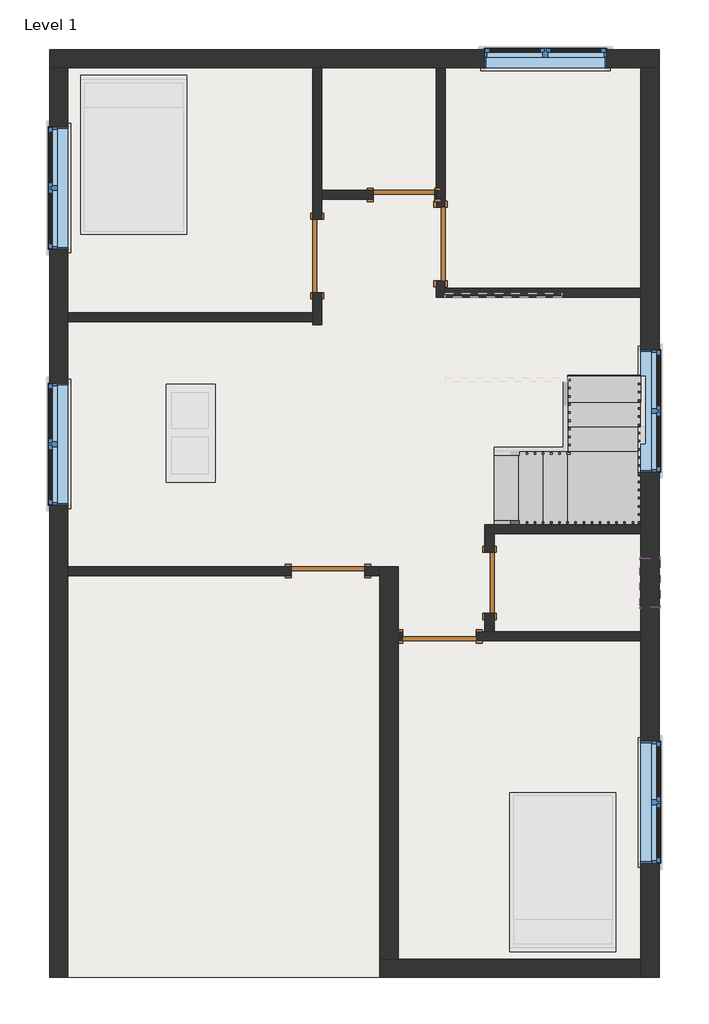
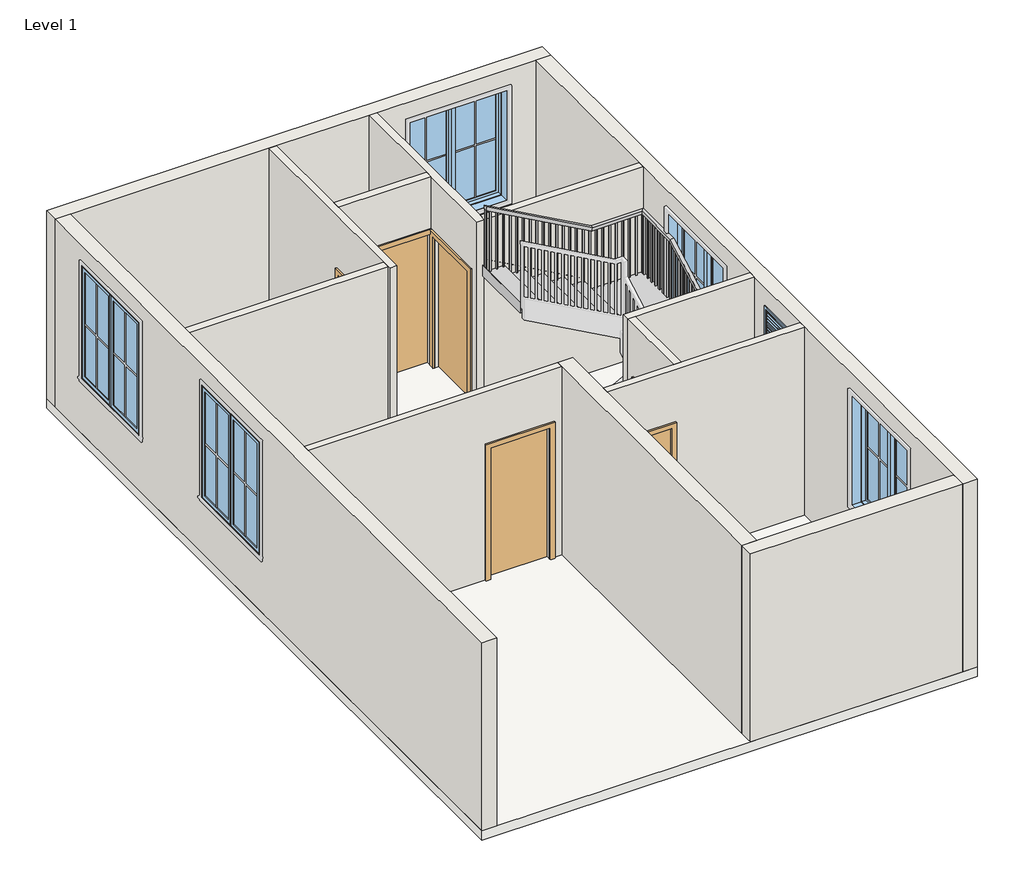
# One storey, part 1 of 2: 14 walls, 6 doors, 6 windows, 1 railing, 1 slab, 1 stair flight.
"""IFC4 building model written with IfcOpenShell, lengths in millimetres."""

from ifc_helpers import new_model, si_unit, frame, origin, origin_with_axes, place, context, project, spatial, polyline, outline, extrude, faceted_brep, transform, mapped, element, save
from components import door_214872d5, door_78caadf7, single_flush_door_3_e5f9f3c4, single_flush_door_3_305aa2a5, stair_flight_7d6782b6, window_casement_double_win_5_f93960c7, window_f2d8fef0

model = new_model("IFC4")

# Units and contexts
model_context = context("Model", 3, world=origin())
ifc_project = project(units=[si_unit("LENGTHUNIT", "METRE", prefix="MILLI")], contexts=[model_context])

# Site, building, storey
site = spatial("IfcSite", under=ifc_project)
building = spatial("IfcBuilding", under=site)
storey = spatial("IfcBuildingStorey", under=building, Name="Level 1", Elevation=0.0)

# Doors
placement = place(None, origin())
door_shape = door_214872d5(model_context)
element("IfcDoor", 1, ObjectType="Single-Flush : DOOR 2'6\"", at=placement, inside=storey, context=model_context, shape_type="MappedRepresentation", body=[
    mapped(door_shape, transform((-185.4325206, 3926.3629493, 0.0), x_axis=(1.0, 0.0, 0.0), y_axis=(0.0, 1.0, 0.0), z_axis=(0.0, 0.0, 1.0))),
])
door_2_shape = door_78caadf7(model_context)
element("IfcDoor", 2, ObjectType="Single-Flush : DOOR 2'6\"", at=placement, inside=storey, context=model_context, shape_type="MappedRepresentation", body=[
    mapped(door_2_shape, transform((881.3674794, -905.9870507, 0.0), x_axis=(0.0, 1.0, 0.0), y_axis=(-1.0, 0.0, 0.0), z_axis=(0.0, 0.0, 1.0))),
])
single_flush_door_3_shape = single_flush_door_3_e5f9f3c4(model_context)
element("IfcDoor", 3, ObjectType="Single-Flush : DOOR 3'", at=placement, inside=storey, context=model_context, shape_type="MappedRepresentation", body=[
    mapped(single_flush_door_3_shape, transform((271.7674794, 3316.7629493, 0.0), x_axis=(0.0, -1.0, 0.0), y_axis=(1.0, 0.0, 0.0), z_axis=(0.0, 0.0, 1.0))),
])
element("IfcDoor", 4, ObjectType="Single-Flush : DOOR 3'", at=placement, inside=storey, context=model_context, shape_type="MappedRepresentation", body=[
    mapped(single_flush_door_3_shape, transform((255.8924794, -1572.7370507, 0.0), x_axis=(-1.0, 0.0, 0.0), y_axis=(0.0, -1.0, 0.0), z_axis=(0.0, 0.0, 1.0))),
])
single_flush_door_3_2_shape = single_flush_door_3_305aa2a5(model_context)
element("IfcDoor", 5, ObjectType="Single-Flush : DOOR 3'", at=placement, inside=storey, context=model_context, shape_type="MappedRepresentation", body=[
    mapped(single_flush_door_3_2_shape, transform((-1264.9325206, 3164.3629493, 0.0), x_axis=(0.0, -1.0, 0.0), y_axis=(1.0, 0.0, 0.0), z_axis=(0.0, 0.0, 1.0))),
])
element("IfcDoor", 6, ObjectType="Single-Flush : DOOR 3'6\"", at=placement, inside=storey, context=model_context, shape_type="MappedRepresentation", body=[
    mapped(single_flush_door_3_shape, transform((-1131.5825206, -759.9370507, 0.0), x_axis=(1.0, 0.0, 0.0), y_axis=(0.0, 1.0, 0.0), z_axis=(0.0, 0.0, 1.0))),
])

# Railing
element("IfcRailing", 7, ObjectType="Handrail - Rectangular", at=placement, inside=storey, context=model_context, shape_type="SolidModel", body=[
    faceted_brep([(938.5174794, -131.2870507, 1083.7333333), (938.5174794, -131.2870507, 1025.620221), (938.5174794, -182.0870507, 1025.620221), (938.5174794, -182.0870507, 1083.7333333), (2005.3174794, -131.2870507, 1676.4), (2018.4810817, -131.2870507, 1625.6), (2018.4810817, -182.0870507, 1625.6), (2005.3174794, -182.0870507, 1676.4), (2716.5174794, -131.2870507, 1676.4), (2716.5174794, -131.2870507, 1625.6), (2767.3174794, -182.0870507, 1625.6), (2767.3174794, -182.0870507, 1676.4), (2716.5174794, 579.9129493, 1676.4), (2716.5174794, 593.0765516, 1625.6), (2767.3174794, 593.0765516, 1625.6), (2767.3174794, 579.9129493, 1676.4), (2716.5174794, 1843.5629493, 2378.4277778), (2716.5174794, 1856.7265516, 2327.6277778), (2767.3174794, 1856.7265516, 2327.6277778), (2767.3174794, 1843.5629493, 2378.4277778), (2716.5174794, 2599.2129493, 2378.4277778), (2716.5174794, 2599.2129493, 2327.6277778), (2767.3174794, 2650.0129493, 2327.6277778), (2767.3174794, 2650.0129493, 2378.4277778), (1960.8674794, 2599.2129493, 2378.4277778), (1947.7038772, 2599.2129493, 2327.6277778), (1947.7038772, 2650.0129493, 2327.6277778), (1960.8674794, 2650.0129493, 2378.4277778), (328.9174794, 2599.2129493, 3285.0666667), (328.9174794, 2650.0129493, 3285.0666667), (328.9174794, 2650.0129493, 3226.9535543), (328.9174794, 2599.2129493, 3226.9535543)], [[[0, 1, 2, 3]], [[1, 0, 4, 5]], [[2, 1, 5, 6]], [[3, 2, 6, 7]], [[0, 3, 7, 4]], [[5, 4, 8, 9]], [[6, 5, 9, 10]], [[7, 6, 10, 11]], [[4, 7, 11, 8]], [[9, 8, 12, 13]], [[10, 9, 13, 14]], [[11, 10, 14, 15]], [[8, 11, 15, 12]], [[13, 12, 16, 17]], [[14, 13, 17, 18]], [[15, 14, 18, 19]], [[12, 15, 19, 16]], [[17, 16, 20, 21]], [[18, 17, 21, 22]], [[19, 18, 22, 23]], [[16, 19, 23, 20]], [[21, 20, 24, 25]], [[22, 21, 25, 26]], [[23, 22, 26, 27]], [[20, 23, 27, 24]], [[28, 29, 30, 31]], [[25, 24, 28, 31]], [[26, 25, 31, 30]], [[27, 26, 30, 29]], [[24, 27, 29, 28]]]),
    extrude(outline(polyline([(3179.3285543, 414.6424794), (3189.9118876, 395.5924794), (2201.3333333, 395.5924794), (2201.3333333, 414.6424794), (3179.3285543, 414.6424794)])), frame((0.0, 2615.0879493, 0.0), z_axis=(0.0, 1.0, 0.0), x_axis=(0.0, 0.0, 1.0)), (0.0, 0.0, 1.0), 19.05),
    extrude(outline(polyline([(3122.8841099, 516.2424794), (3133.4674432, 497.1924794), (2201.3333333, 497.1924794), (2201.3333333, 516.2424794), (3122.8841099, 516.2424794)])), frame((0.0, 2615.0879493, 0.0), z_axis=(0.0, 1.0, 0.0), x_axis=(0.0, 0.0, 1.0)), (0.0, 0.0, 1.0), 19.05),
    extrude(outline(polyline([(3066.4396654, 617.8424794), (3077.0229988, 598.7924794), (2201.3333333, 598.7924794), (2201.3333333, 617.8424794), (3066.4396654, 617.8424794)])), frame((0.0, 2615.0879493, 0.0), z_axis=(0.0, 1.0, 0.0), x_axis=(0.0, 0.0, 1.0)), (0.0, 0.0, 1.0), 19.05),
    extrude(outline(polyline([(3009.995221, 719.4424794), (3020.5785543, 700.3924794), (2032.0, 700.3924794), (2032.0, 719.4424794), (3009.995221, 719.4424794)])), frame((0.0, 2615.0879493, 0.0), z_axis=(0.0, 1.0, 0.0), x_axis=(0.0, 0.0, 1.0)), (0.0, 0.0, 1.0), 19.05),
    extrude(outline(polyline([(2953.5507765, 821.0424794), (2964.1341099, 801.9924794), (2032.0, 801.9924794), (2032.0, 821.0424794), (2953.5507765, 821.0424794)])), frame((0.0, 2615.0879493, 0.0), z_axis=(0.0, 1.0, 0.0), x_axis=(0.0, 0.0, 1.0)), (0.0, 0.0, 1.0), 19.05),
    extrude(outline(polyline([(2897.1063321, 922.6424794), (2907.6896654, 903.5924794), (2032.0, 903.5924794), (2032.0, 922.6424794), (2897.1063321, 922.6424794)])), frame((0.0, 2615.0879493, 0.0), z_axis=(0.0, 1.0, 0.0), x_axis=(0.0, 0.0, 1.0)), (0.0, 0.0, 1.0), 19.05),
    extrude(outline(polyline([(2840.6618876, 1024.2424794), (2851.245221, 1005.1924794), (1862.6666667, 1005.1924794), (1862.6666667, 1024.2424794), (2840.6618876, 1024.2424794)])), frame((0.0, 2615.0879493, 0.0), z_axis=(0.0, 1.0, 0.0), x_axis=(0.0, 0.0, 1.0)), (0.0, 0.0, 1.0), 19.05),
    extrude(outline(polyline([(2784.2174432, 1125.8424794), (2794.8007765, 1106.7924794), (1862.6666667, 1106.7924794), (1862.6666667, 1125.8424794), (2784.2174432, 1125.8424794)])), frame((0.0, 2615.0879493, 0.0), z_axis=(0.0, 1.0, 0.0), x_axis=(0.0, 0.0, 1.0)), (0.0, 0.0, 1.0), 19.05),
    extrude(outline(polyline([(2727.7729988, 1227.4424794), (2738.3563321, 1208.3924794), (1862.6666667, 1208.3924794), (1862.6666667, 1227.4424794), (2727.7729988, 1227.4424794)])), frame((0.0, 2615.0879493, 0.0), z_axis=(0.0, 1.0, 0.0), x_axis=(0.0, 0.0, 1.0)), (0.0, 0.0, 1.0), 19.05),
    extrude(outline(polyline([(2671.3285543, 1329.0424794), (2681.9118876, 1309.9924794), (1693.3333333, 1309.9924794), (1693.3333333, 1329.0424794), (2671.3285543, 1329.0424794)])), frame((0.0, 2615.0879493, 0.0), z_axis=(0.0, 1.0, 0.0), x_axis=(0.0, 0.0, 1.0)), (0.0, 0.0, 1.0), 19.05),
    extrude(outline(polyline([(2614.8841099, 1430.6424794), (2625.4674432, 1411.5924794), (1693.3333333, 1411.5924794), (1693.3333333, 1430.6424794), (2614.8841099, 1430.6424794)])), frame((0.0, 2615.0879493, 0.0), z_axis=(0.0, 1.0, 0.0), x_axis=(0.0, 0.0, 1.0)), (0.0, 0.0, 1.0), 19.05),
    extrude(outline(polyline([(2558.4396654, 1532.2424794), (2569.0229988, 1513.1924794), (1693.3333333, 1513.1924794), (1693.3333333, 1532.2424794), (2558.4396654, 1532.2424794)])), frame((0.0, 2615.0879493, 0.0), z_axis=(0.0, 1.0, 0.0), x_axis=(0.0, 0.0, 1.0)), (0.0, 0.0, 1.0), 19.05),
    extrude(outline(polyline([(2501.995221, 1633.8424794), (2512.5785543, 1614.7924794), (1524.0, 1614.7924794), (1524.0, 1633.8424794), (2501.995221, 1633.8424794)])), frame((0.0, 2615.0879493, 0.0), z_axis=(0.0, 1.0, 0.0), x_axis=(0.0, 0.0, 1.0)), (0.0, 0.0, 1.0), 19.05),
    extrude(outline(polyline([(2445.5507765, 1735.4424794), (2456.1341099, 1716.3924794), (1524.0, 1716.3924794), (1524.0, 1735.4424794), (2445.5507765, 1735.4424794)])), frame((0.0, 2615.0879493, 0.0), z_axis=(0.0, 1.0, 0.0), x_axis=(0.0, 0.0, 1.0)), (0.0, 0.0, 1.0), 19.05),
    extrude(outline(polyline([(2389.1063321, 1837.0424794), (2399.6896654, 1817.9924794), (1524.0, 1817.9924794), (1524.0, 1837.0424794), (2389.1063321, 1837.0424794)])), frame((0.0, 2615.0879493, 0.0), z_axis=(0.0, 1.0, 0.0), x_axis=(0.0, 0.0, 1.0)), (0.0, 0.0, 1.0), 19.05),
    extrude(outline(polyline([(2332.6618876, 1938.6424794), (2343.245221, 1919.5924794), (1354.6666667, 1919.5924794), (1354.6666667, 1938.6424794), (2332.6618876, 1938.6424794)])), frame((0.0, 2615.0879493, 0.0), z_axis=(0.0, 1.0, 0.0), x_axis=(0.0, 0.0, 1.0)), (0.0, 0.0, 1.0), 19.05),
    extrude(outline(polyline([(2040.2424794, 2634.1379493), (2040.2424794, 2615.0879493), (2021.1924794, 2615.0879493), (2021.1924794, 2634.1379493), (2040.2424794, 2634.1379493)])), frame((0.0, 0.0, 1354.6666667), z_axis=(0.0, 0.0, 1.0), x_axis=(1.0, 0.0, 0.0)), (0.0, 0.0, 1.0), 972.9611111),
    extrude(outline(polyline([(2141.8424794, 2634.1379493), (2141.8424794, 2615.0879493), (2122.7924794, 2615.0879493), (2122.7924794, 2634.1379493), (2141.8424794, 2634.1379493)])), frame((0.0, 0.0, 1354.6666667), z_axis=(0.0, 0.0, 1.0), x_axis=(1.0, 0.0, 0.0)), (0.0, 0.0, 1.0), 972.9611111),
    extrude(outline(polyline([(2243.4424794, 2634.1379493), (2243.4424794, 2615.0879493), (2224.3924794, 2615.0879493), (2224.3924794, 2634.1379493), (2243.4424794, 2634.1379493)])), frame((0.0, 0.0, 1354.6666667), z_axis=(0.0, 0.0, 1.0), x_axis=(1.0, 0.0, 0.0)), (0.0, 0.0, 1.0), 972.9611111),
    extrude(outline(polyline([(2345.0424794, 2634.1379493), (2345.0424794, 2615.0879493), (2325.9924794, 2615.0879493), (2325.9924794, 2634.1379493), (2345.0424794, 2634.1379493)])), frame((0.0, 0.0, 1354.6666667), z_axis=(0.0, 0.0, 1.0), x_axis=(1.0, 0.0, 0.0)), (0.0, 0.0, 1.0), 972.9611111),
    extrude(outline(polyline([(2446.6424794, 2634.1379493), (2446.6424794, 2615.0879493), (2427.5924794, 2615.0879493), (2427.5924794, 2634.1379493), (2446.6424794, 2634.1379493)])), frame((0.0, 0.0, 1354.6666667), z_axis=(0.0, 0.0, 1.0), x_axis=(1.0, 0.0, 0.0)), (0.0, 0.0, 1.0), 972.9611111),
    extrude(outline(polyline([(2548.2424794, 2634.1379493), (2548.2424794, 2615.0879493), (2529.1924794, 2615.0879493), (2529.1924794, 2634.1379493), (2548.2424794, 2634.1379493)])), frame((0.0, 0.0, 1354.6666667), z_axis=(0.0, 0.0, 1.0), x_axis=(1.0, 0.0, 0.0)), (0.0, 0.0, 1.0), 972.9611111),
    extrude(outline(polyline([(2649.8424794, 2634.1379493), (2649.8424794, 2615.0879493), (2630.7924794, 2615.0879493), (2630.7924794, 2634.1379493), (2649.8424794, 2634.1379493)])), frame((0.0, 0.0, 1354.6666667), z_axis=(0.0, 0.0, 1.0), x_axis=(1.0, 0.0, 0.0)), (0.0, 0.0, 1.0), 972.9611111),
    extrude(outline(polyline([(2751.4424794, 2576.9879493), (2732.3924794, 2576.9879493), (2732.3924794, 2596.0379493), (2751.4424794, 2596.0379493), (2751.4424794, 2576.9879493)])), frame((0.0, 0.0, 1354.6666667), z_axis=(0.0, 0.0, 1.0), x_axis=(1.0, 0.0, 0.0)), (0.0, 0.0, 1.0), 972.9611111),
    extrude(outline(polyline([(2751.4424794, 2475.3879493), (2732.3924794, 2475.3879493), (2732.3924794, 2494.4379493), (2751.4424794, 2494.4379493), (2751.4424794, 2475.3879493)])), frame((0.0, 0.0, 1354.6666667), z_axis=(0.0, 0.0, 1.0), x_axis=(1.0, 0.0, 0.0)), (0.0, 0.0, 1.0), 972.9611111),
    extrude(outline(polyline([(2751.4424794, 2373.7879493), (2732.3924794, 2373.7879493), (2732.3924794, 2392.8379493), (2751.4424794, 2392.8379493), (2751.4424794, 2373.7879493)])), frame((0.0, 0.0, 1354.6666667), z_axis=(0.0, 0.0, 1.0), x_axis=(1.0, 0.0, 0.0)), (0.0, 0.0, 1.0), 972.9611111),
    extrude(outline(polyline([(2751.4424794, 2272.1879493), (2732.3924794, 2272.1879493), (2732.3924794, 2291.2379493), (2751.4424794, 2291.2379493), (2751.4424794, 2272.1879493)])), frame((0.0, 0.0, 1354.6666667), z_axis=(0.0, 0.0, 1.0), x_axis=(1.0, 0.0, 0.0)), (0.0, 0.0, 1.0), 972.9611111),
    extrude(outline(polyline([(2751.4424794, 2170.5879493), (2732.3924794, 2170.5879493), (2732.3924794, 2189.6379493), (2751.4424794, 2189.6379493), (2751.4424794, 2170.5879493)])), frame((0.0, 0.0, 1354.6666667), z_axis=(0.0, 0.0, 1.0), x_axis=(1.0, 0.0, 0.0)), (0.0, 0.0, 1.0), 972.9611111),
    extrude(outline(polyline([(2751.4424794, 2068.9879493), (2732.3924794, 2068.9879493), (2732.3924794, 2088.0379493), (2751.4424794, 2088.0379493), (2751.4424794, 2068.9879493)])), frame((0.0, 0.0, 1354.6666667), z_axis=(0.0, 0.0, 1.0), x_axis=(1.0, 0.0, 0.0)), (0.0, 0.0, 1.0), 972.9611111),
    extrude(outline(polyline([(2751.4424794, 1967.3879493), (2732.3924794, 1967.3879493), (2732.3924794, 1986.4379493), (2751.4424794, 1986.4379493), (2751.4424794, 1967.3879493)])), frame((0.0, 0.0, 1354.6666667), z_axis=(0.0, 0.0, 1.0), x_axis=(1.0, 0.0, 0.0)), (0.0, 0.0, 1.0), 972.9611111),
    extrude(outline(polyline([(2751.4424794, 1865.7879493), (2732.3924794, 1865.7879493), (2732.3924794, 1884.8379493), (2751.4424794, 1884.8379493), (2751.4424794, 1865.7879493)])), frame((0.0, 0.0, 1354.6666667), z_axis=(0.0, 0.0, 1.0), x_axis=(1.0, 0.0, 0.0)), (0.0, 0.0, 1.0), 972.9611111),
    extrude(outline(polyline([(1764.1879493, 2276.2174432), (1783.2379493, 2286.8007765), (1783.2379493, 1354.6666667), (1764.1879493, 1354.6666667), (1764.1879493, 2276.2174432)])), frame((2732.3924794, 0.0, 0.0), z_axis=(1.0, 0.0, 0.0), x_axis=(0.0, 1.0, 0.0)), (0.0, 0.0, 1.0), 19.05),
    extrude(outline(polyline([(1662.5879493, 2219.7729988), (1681.6379493, 2230.3563321), (1681.6379493, 1354.6666667), (1662.5879493, 1354.6666667), (1662.5879493, 2219.7729988)])), frame((2732.3924794, 0.0, 0.0), z_axis=(1.0, 0.0, 0.0), x_axis=(0.0, 1.0, 0.0)), (0.0, 0.0, 1.0), 19.05),
    extrude(outline(polyline([(1560.9879493, 2163.3285543), (1580.0379493, 2173.9118876), (1580.0379493, 1185.3333333), (1560.9879493, 1185.3333333), (1560.9879493, 2163.3285543)])), frame((2732.3924794, 0.0, 0.0), z_axis=(1.0, 0.0, 0.0), x_axis=(0.0, 1.0, 0.0)), (0.0, 0.0, 1.0), 19.05),
    extrude(outline(polyline([(1459.3879493, 2106.8841099), (1478.4379493, 2117.4674432), (1478.4379493, 1185.3333333), (1459.3879493, 1185.3333333), (1459.3879493, 2106.8841099)])), frame((2732.3924794, 0.0, 0.0), z_axis=(1.0, 0.0, 0.0), x_axis=(0.0, 1.0, 0.0)), (0.0, 0.0, 1.0), 19.05),
    extrude(outline(polyline([(1357.7879493, 2050.4396654), (1376.8379493, 2061.0229988), (1376.8379493, 1185.3333333), (1357.7879493, 1185.3333333), (1357.7879493, 2050.4396654)])), frame((2732.3924794, 0.0, 0.0), z_axis=(1.0, 0.0, 0.0), x_axis=(0.0, 1.0, 0.0)), (0.0, 0.0, 1.0), 19.05),
    extrude(outline(polyline([(1256.1879493, 1993.995221), (1275.2379493, 2004.5785543), (1275.2379493, 1016.0), (1256.1879493, 1016.0), (1256.1879493, 1993.995221)])), frame((2732.3924794, 0.0, 0.0), z_axis=(1.0, 0.0, 0.0), x_axis=(0.0, 1.0, 0.0)), (0.0, 0.0, 1.0), 19.05),
    extrude(outline(polyline([(1154.5879493, 1937.5507765), (1173.6379493, 1948.1341099), (1173.6379493, 1016.0), (1154.5879493, 1016.0), (1154.5879493, 1937.5507765)])), frame((2732.3924794, 0.0, 0.0), z_axis=(1.0, 0.0, 0.0), x_axis=(0.0, 1.0, 0.0)), (0.0, 0.0, 1.0), 19.05),
    extrude(outline(polyline([(1052.9879493, 1881.1063321), (1072.0379493, 1891.6896654), (1072.0379493, 1016.0), (1052.9879493, 1016.0), (1052.9879493, 1881.1063321)])), frame((2732.3924794, 0.0, 0.0), z_axis=(1.0, 0.0, 0.0), x_axis=(0.0, 1.0, 0.0)), (0.0, 0.0, 1.0), 19.05),
    extrude(outline(polyline([(951.3879493, 1824.6618876), (970.4379493, 1835.245221), (970.4379493, 846.6666667), (951.3879493, 846.6666667), (951.3879493, 1824.6618876)])), frame((2732.3924794, 0.0, 0.0), z_axis=(1.0, 0.0, 0.0), x_axis=(0.0, 1.0, 0.0)), (0.0, 0.0, 1.0), 19.05),
    extrude(outline(polyline([(849.7879493, 1768.2174432), (868.8379493, 1778.8007765), (868.8379493, 846.6666667), (849.7879493, 846.6666667), (849.7879493, 1768.2174432)])), frame((2732.3924794, 0.0, 0.0), z_axis=(1.0, 0.0, 0.0), x_axis=(0.0, 1.0, 0.0)), (0.0, 0.0, 1.0), 19.05),
    extrude(outline(polyline([(748.1879493, 1711.7729988), (767.2379493, 1722.3563321), (767.2379493, 846.6666667), (748.1879493, 846.6666667), (748.1879493, 1711.7729988)])), frame((2732.3924794, 0.0, 0.0), z_axis=(1.0, 0.0, 0.0), x_axis=(0.0, 1.0, 0.0)), (0.0, 0.0, 1.0), 19.05),
    extrude(outline(polyline([(646.5879493, 1655.3285543), (665.6379493, 1665.9118876), (665.6379493, 677.3333333), (646.5879493, 677.3333333), (646.5879493, 1655.3285543)])), frame((2732.3924794, 0.0, 0.0), z_axis=(1.0, 0.0, 0.0), x_axis=(0.0, 1.0, 0.0)), (0.0, 0.0, 1.0), 19.05),
    extrude(outline(polyline([(2751.4424794, 544.9879493), (2732.3924794, 544.9879493), (2732.3924794, 564.0379493), (2751.4424794, 564.0379493), (2751.4424794, 544.9879493)])), frame((0.0, 0.0, 677.3333333), z_axis=(0.0, 0.0, 1.0), x_axis=(1.0, 0.0, 0.0)), (0.0, 0.0, 1.0), 948.2666667),
    extrude(outline(polyline([(2751.4424794, 443.3879493), (2732.3924794, 443.3879493), (2732.3924794, 462.4379493), (2751.4424794, 462.4379493), (2751.4424794, 443.3879493)])), frame((0.0, 0.0, 677.3333333), z_axis=(0.0, 0.0, 1.0), x_axis=(1.0, 0.0, 0.0)), (0.0, 0.0, 1.0), 948.2666667),
    extrude(outline(polyline([(2751.4424794, 341.7879493), (2732.3924794, 341.7879493), (2732.3924794, 360.8379493), (2751.4424794, 360.8379493), (2751.4424794, 341.7879493)])), frame((0.0, 0.0, 677.3333333), z_axis=(0.0, 0.0, 1.0), x_axis=(1.0, 0.0, 0.0)), (0.0, 0.0, 1.0), 948.2666667),
    extrude(outline(polyline([(2751.4424794, 240.1879493), (2732.3924794, 240.1879493), (2732.3924794, 259.2379493), (2751.4424794, 259.2379493), (2751.4424794, 240.1879493)])), frame((0.0, 0.0, 677.3333333), z_axis=(0.0, 0.0, 1.0), x_axis=(1.0, 0.0, 0.0)), (0.0, 0.0, 1.0), 948.2666667),
    extrude(outline(polyline([(2751.4424794, 138.5879493), (2732.3924794, 138.5879493), (2732.3924794, 157.6379493), (2751.4424794, 157.6379493), (2751.4424794, 138.5879493)])), frame((0.0, 0.0, 677.3333333), z_axis=(0.0, 0.0, 1.0), x_axis=(1.0, 0.0, 0.0)), (0.0, 0.0, 1.0), 948.2666667),
    extrude(outline(polyline([(2751.4424794, 36.9879493), (2732.3924794, 36.9879493), (2732.3924794, 56.0379493), (2751.4424794, 56.0379493), (2751.4424794, 36.9879493)])), frame((0.0, 0.0, 677.3333333), z_axis=(0.0, 0.0, 1.0), x_axis=(1.0, 0.0, 0.0)), (0.0, 0.0, 1.0), 948.2666667),
    extrude(outline(polyline([(2751.4424794, -64.6120507), (2732.3924794, -64.6120507), (2732.3924794, -45.5620507), (2751.4424794, -45.5620507), (2751.4424794, -64.6120507)])), frame((0.0, 0.0, 677.3333333), z_axis=(0.0, 0.0, 1.0), x_axis=(1.0, 0.0, 0.0)), (0.0, 0.0, 1.0), 948.2666667),
    extrude(outline(polyline([(2656.1924794, -166.2120507), (2656.1924794, -147.1620507), (2675.2424794, -147.1620507), (2675.2424794, -166.2120507), (2656.1924794, -166.2120507)])), frame((0.0, 0.0, 677.3333333), z_axis=(0.0, 0.0, 1.0), x_axis=(1.0, 0.0, 0.0)), (0.0, 0.0, 1.0), 948.2666667),
    extrude(outline(polyline([(2554.5924794, -166.2120507), (2554.5924794, -147.1620507), (2573.6424794, -147.1620507), (2573.6424794, -166.2120507), (2554.5924794, -166.2120507)])), frame((0.0, 0.0, 677.3333333), z_axis=(0.0, 0.0, 1.0), x_axis=(1.0, 0.0, 0.0)), (0.0, 0.0, 1.0), 948.2666667),
    extrude(outline(polyline([(2452.9924794, -166.2120507), (2452.9924794, -147.1620507), (2472.0424794, -147.1620507), (2472.0424794, -166.2120507), (2452.9924794, -166.2120507)])), frame((0.0, 0.0, 677.3333333), z_axis=(0.0, 0.0, 1.0), x_axis=(1.0, 0.0, 0.0)), (0.0, 0.0, 1.0), 948.2666667),
    extrude(outline(polyline([(2351.3924794, -166.2120507), (2351.3924794, -147.1620507), (2370.4424794, -147.1620507), (2370.4424794, -166.2120507), (2351.3924794, -166.2120507)])), frame((0.0, 0.0, 677.3333333), z_axis=(0.0, 0.0, 1.0), x_axis=(1.0, 0.0, 0.0)), (0.0, 0.0, 1.0), 948.2666667),
    extrude(outline(polyline([(2249.7924794, -166.2120507), (2249.7924794, -147.1620507), (2268.8424794, -147.1620507), (2268.8424794, -166.2120507), (2249.7924794, -166.2120507)])), frame((0.0, 0.0, 677.3333333), z_axis=(0.0, 0.0, 1.0), x_axis=(1.0, 0.0, 0.0)), (0.0, 0.0, 1.0), 948.2666667),
    extrude(outline(polyline([(2148.1924794, -166.2120507), (2148.1924794, -147.1620507), (2167.2424794, -147.1620507), (2167.2424794, -166.2120507), (2148.1924794, -166.2120507)])), frame((0.0, 0.0, 677.3333333), z_axis=(0.0, 0.0, 1.0), x_axis=(1.0, 0.0, 0.0)), (0.0, 0.0, 1.0), 948.2666667),
    extrude(outline(polyline([(2046.5924794, -166.2120507), (2046.5924794, -147.1620507), (2065.6424794, -147.1620507), (2065.6424794, -166.2120507), (2046.5924794, -166.2120507)])), frame((0.0, 0.0, 677.3333333), z_axis=(0.0, 0.0, 1.0), x_axis=(1.0, 0.0, 0.0)), (0.0, 0.0, 1.0), 948.2666667),
    extrude(outline(polyline([(1595.3563321, 1964.0424794), (1584.7729988, 1944.9924794), (677.3333333, 1944.9924794), (677.3333333, 1964.0424794), (1595.3563321, 1964.0424794)])), frame((0.0, -166.2120507, 0.0), z_axis=(0.0, 1.0, 0.0), x_axis=(0.0, 0.0, 1.0)), (0.0, 0.0, 1.0), 19.05),
    extrude(outline(polyline([(1538.9118876, 1862.4424794), (1528.3285543, 1843.3924794), (677.3333333, 1843.3924794), (677.3333333, 1862.4424794), (1538.9118876, 1862.4424794)])), frame((0.0, -166.2120507, 0.0), z_axis=(0.0, 1.0, 0.0), x_axis=(0.0, 0.0, 1.0)), (0.0, 0.0, 1.0), 19.05),
    extrude(outline(polyline([(1482.4674432, 1760.8424794), (1471.8841099, 1741.7924794), (508.0, 1741.7924794), (508.0, 1760.8424794), (1482.4674432, 1760.8424794)])), frame((0.0, -166.2120507, 0.0), z_axis=(0.0, 1.0, 0.0), x_axis=(0.0, 0.0, 1.0)), (0.0, 0.0, 1.0), 19.05),
    extrude(outline(polyline([(1426.0229988, 1659.2424794), (1415.4396654, 1640.1924794), (508.0, 1640.1924794), (508.0, 1659.2424794), (1426.0229988, 1659.2424794)])), frame((0.0, -166.2120507, 0.0), z_axis=(0.0, 1.0, 0.0), x_axis=(0.0, 0.0, 1.0)), (0.0, 0.0, 1.0), 19.05),
    extrude(outline(polyline([(1369.5785543, 1557.6424794), (1358.995221, 1538.5924794), (508.0, 1538.5924794), (508.0, 1557.6424794), (1369.5785543, 1557.6424794)])), frame((0.0, -166.2120507, 0.0), z_axis=(0.0, 1.0, 0.0), x_axis=(0.0, 0.0, 1.0)), (0.0, 0.0, 1.0), 19.05),
    extrude(outline(polyline([(1313.1341099, 1456.0424794), (1302.5507765, 1436.9924794), (338.6666667, 1436.9924794), (338.6666667, 1456.0424794), (1313.1341099, 1456.0424794)])), frame((0.0, -166.2120507, 0.0), z_axis=(0.0, 1.0, 0.0), x_axis=(0.0, 0.0, 1.0)), (0.0, 0.0, 1.0), 19.05),
    extrude(outline(polyline([(1256.6896654, 1354.4424794), (1246.1063321, 1335.3924794), (338.6666667, 1335.3924794), (338.6666667, 1354.4424794), (1256.6896654, 1354.4424794)])), frame((0.0, -166.2120507, 0.0), z_axis=(0.0, 1.0, 0.0), x_axis=(0.0, 0.0, 1.0)), (0.0, 0.0, 1.0), 19.05),
    extrude(outline(polyline([(1200.245221, 1252.8424794), (1189.6618876, 1233.7924794), (338.6666667, 1233.7924794), (338.6666667, 1252.8424794), (1200.245221, 1252.8424794)])), frame((0.0, -166.2120507, 0.0), z_axis=(0.0, 1.0, 0.0), x_axis=(0.0, 0.0, 1.0)), (0.0, 0.0, 1.0), 19.05),
    extrude(outline(polyline([(1143.8007765, 1151.2424794), (1133.2174432, 1132.1924794), (169.3333333, 1132.1924794), (169.3333333, 1151.2424794), (1143.8007765, 1151.2424794)])), frame((0.0, -166.2120507, 0.0), z_axis=(0.0, 1.0, 0.0), x_axis=(0.0, 0.0, 1.0)), (0.0, 0.0, 1.0), 19.05),
    extrude(outline(polyline([(1087.3563321, 1049.6424794), (1076.7729988, 1030.5924794), (169.3333333, 1030.5924794), (169.3333333, 1049.6424794), (1087.3563321, 1049.6424794)])), frame((0.0, -166.2120507, 0.0), z_axis=(0.0, 1.0, 0.0), x_axis=(0.0, 0.0, 1.0)), (0.0, 0.0, 1.0), 19.05),
    extrude(outline(polyline([(2751.4424794, 2615.0879493), (2732.3924794, 2615.0879493), (2732.3924794, 2634.1379493), (2751.4424794, 2634.1379493), (2751.4424794, 2615.0879493)])), frame((0.0, 0.0, 1354.6666667), z_axis=(0.0, 0.0, 1.0), x_axis=(1.0, 0.0, 0.0)), (0.0, 0.0, 1.0), 972.9611111),
    extrude(outline(polyline([(2732.3924794, -166.2120507), (2732.3924794, -147.1620507), (2751.4424794, -147.1620507), (2751.4424794, -166.2120507), (2732.3924794, -166.2120507)])), frame((0.0, 0.0, 677.3333333), z_axis=(0.0, 0.0, 1.0), x_axis=(1.0, 0.0, 0.0)), (0.0, 0.0, 1.0), 948.2666667),
    extrude(outline(polyline([(3216.370221, 347.9674794), (3226.9535543, 328.9174794), (2201.3333333, 328.9174794), (2201.3333333, 347.9674794), (3216.370221, 347.9674794)])), frame((0.0, 2615.0879493, 0.0), z_axis=(0.0, 1.0, 0.0), x_axis=(0.0, 0.0, 1.0)), (0.0, 0.0, 1.0), 19.05),
    extrude(outline(polyline([(1036.2035543, 957.5674794), (1025.620221, 938.5174794), (169.3333333, 938.5174794), (169.3333333, 957.5674794), (1036.2035543, 957.5674794)])), frame((0.0, -166.2120507, 0.0), z_axis=(0.0, 1.0, 0.0), x_axis=(0.0, 0.0, 1.0)), (0.0, 0.0, 1.0), 19.05),
])

# Slab
element("IfcSlab", 8, ObjectType="FLOOR 6\"", at=placement, inside=storey, context=model_context, shape_type="SweptSolid", body=[
    extrude(outline(polyline([(2995.9174794, 5736.1129493), (2995.9174794, -5820.8870507), (-4598.6825206, -5820.8870507), (-4598.6825206, 5736.1129493), (2995.9174794, 5736.1129493)])), frame((0.0, 0.0, -152.4), z_axis=(0.0, 0.0, 1.0), x_axis=(1.0, 0.0, 0.0)), (0.0, 0.0, 1.0), 152.4),
])

# Stair flight
stair_flight_shape = stair_flight_7d6782b6(model_context)
element("IfcStairFlight", 9, ObjectType="2\" Tread 1\" Nosing 1/4\" Riser", at=placement, inside=storey, context=model_context, shape_type="MappedRepresentation", body=[
    mapped(stair_flight_shape, transform((0.0, 0.0, 0.0), x_axis=(1.0, 0.0, 0.0), y_axis=(0.0, 1.0, 0.0), z_axis=(0.0, 0.0, 1.0))),
])

# Walls
element("IfcWall", 10, at=placement, inside=storey, context=model_context, shape_type="Brep", body=[
    faceted_brep([(-1322.0825206, 2707.1629493, 2133.6), (-1322.0825206, 2707.1629493, 0.0), (-1322.0825206, 2459.5129493, 0.0), (-1322.0825206, 2345.2129493, 0.0), (-1322.0825206, 2307.1129493, 0.0), (-1322.0825206, 2307.1129493, 3048.0), (-1322.0825206, 2345.2129493, 3048.0), (-1322.0825206, 2459.5129493, 3048.0), (-1322.0825206, 5507.5129493, 3048.0), (-1322.0825206, 5507.5129493, 0.0), (-1322.0825206, 3621.5629493, 0.0), (-1322.0825206, 3621.5629493, 2133.6), (-1207.7825206, 2307.1129493, 0.0), (-1207.7825206, 2707.1629493, 0.0), (-1207.7825206, 2707.1629493, 2133.6), (-1207.7825206, 3621.5629493, 2133.6), (-1207.7825206, 3621.5629493, 0.0), (-1207.7825206, 3869.2129493, 0.0), (-1207.7825206, 3983.5129493, 0.0), (-1207.7825206, 5507.5129493, 0.0), (-1207.7825206, 5507.5129493, 3048.0), (-1207.7825206, 3983.5129493, 3048.0), (-1207.7825206, 3869.2129493, 3048.0), (-1207.7825206, 2307.1129493, 3048.0)], [[[0, 1, 2, 3, 4, 5, 6, 7, 8, 9, 10, 11]], [[12, 13, 14, 15, 16, 17, 18, 19, 20, 21, 22, 23]], [[10, 9, 19, 18, 17, 16]], [[4, 3, 2, 1, 13, 12]], [[5, 4, 12, 23]], [[9, 8, 20, 19]], [[14, 13, 1, 0]], [[15, 14, 0, 11]], [[16, 15, 11, 10]], [[8, 7, 6, 5, 23, 22, 21, 20]]]),
])
element("IfcWall", 11, at=placement, inside=storey, context=model_context, shape_type="SweptSolid", body=[
    extrude(outline(polyline([(-1322.0825206, 2345.2129493), (-4370.0825206, 2345.2129493), (-4370.0825206, 2459.5129493), (-1322.0825206, 2459.5129493), (-1322.0825206, 2345.2129493)])), origin_with_axes(), (0.0, 0.0, 1.0), 3048.0),
])
element("IfcWall", 12, at=placement, inside=storey, context=model_context, shape_type="SweptSolid", body=[
    extrude(outline(polyline([(2133.6, 195.5674794), (0.0, 195.5674794), (0.0, 214.6174794), (3048.0, 214.6174794), (3048.0, -1207.7825206), (0.0, -1207.7825206), (0.0, -566.4325206), (2133.6, -566.4325206), (2133.6, 195.5674794)])), frame((0.0, 3869.2129493, 0.0), z_axis=(0.0, 1.0, 0.0), x_axis=(0.0, 0.0, 1.0)), (0.0, 0.0, 1.0), 114.3),
])
element("IfcWall", 13, at=placement, inside=storey, context=model_context, shape_type="Brep", body=[
    faceted_brep([(214.6174794, 2859.5629493, 2133.6), (214.6174794, 2859.5629493, 0.0), (214.6174794, 2650.0129493, 0.0), (214.6174794, 2650.0129493, 3048.0), (214.6174794, 3869.2129493, 3048.0), (214.6174794, 3983.5129493, 3048.0), (214.6174794, 5507.5129493, 3048.0), (214.6174794, 5507.5129493, 0.0), (214.6174794, 3983.5129493, 0.0), (214.6174794, 3869.2129493, 0.0), (214.6174794, 3773.9629493, 0.0), (214.6174794, 3773.9629493, 2133.6), (328.9174794, 2650.0129493, 0.0), (328.9174794, 2764.3129493, 0.0), (328.9174794, 2859.5629493, 0.0), (328.9174794, 2859.5629493, 2133.6), (328.9174794, 3773.9629493, 2133.6), (328.9174794, 3773.9629493, 0.0), (328.9174794, 5507.5129493, 0.0), (328.9174794, 5507.5129493, 3048.0), (328.9174794, 2764.3129493, 3048.0), (328.9174794, 2650.0129493, 3048.0)], [[[0, 1, 2, 3, 4, 5, 6, 7, 8, 9, 10, 11]], [[12, 13, 14, 15, 16, 17, 18, 19, 20, 21]], [[2, 1, 14, 13, 12]], [[10, 9, 8, 7, 18, 17]], [[7, 6, 19, 18]], [[3, 2, 12, 21]], [[15, 14, 1, 0]], [[16, 15, 0, 11]], [[17, 16, 11, 10]], [[6, 5, 4, 3, 21, 20, 19]]]),
])
element("IfcWall", 14, at=placement, inside=storey, context=model_context, shape_type="SweptSolid", body=[
    extrude(outline(polyline([(2767.3174794, 2650.0129493), (328.9174794, 2650.0129493), (328.9174794, 2764.3129493), (2767.3174794, 2764.3129493), (2767.3174794, 2650.0129493)])), origin_with_axes(), (0.0, 0.0, 1.0), 3048.0),
])
element("IfcWall", 15, at=placement, inside=storey, context=model_context, shape_type="Brep", body=[
    faceted_brep([(2767.3174794, -182.0870507, 0.0), (824.2174794, -182.0870507, 0.0), (824.2174794, -182.0870507, 3048.0), (2767.3174794, -182.0870507, 3048.0), (2767.3174794, -296.3870507, 0.0), (2767.3174794, -296.3870507, 3048.0), (938.5174794, -296.3870507, 3048.0), (824.2174794, -296.3870507, 3048.0), (824.2174794, -296.3870507, 0.0), (938.5174794, -296.3870507, 0.0)], [[[0, 1, 2, 3]], [[4, 5, 6, 7, 8, 9]], [[1, 0, 4, 9, 8]], [[0, 3, 5, 4]], [[2, 1, 8, 7]], [[3, 2, 7, 6, 5]]]),
])
element("IfcWall", 16, at=placement, inside=storey, context=model_context, shape_type="SweptSolid", body=[
    extrude(outline(polyline([(-296.3870507, 0.0), (-524.9870507, 0.0), (-524.9870507, 2133.6), (-1286.9870507, 2133.6), (-1286.9870507, 0.0), (-1515.5870507, 0.0), (-1515.5870507, 3048.0), (-296.3870507, 3048.0), (-296.3870507, 0.0)])), frame((824.2174794, 0.0, 0.0), z_axis=(1.0, 0.0, 0.0), x_axis=(0.0, 1.0, 0.0)), (0.0, 0.0, 1.0), 114.3),
])
element("IfcWall", 17, at=placement, inside=storey, context=model_context, shape_type="Brep", body=[
    faceted_brep([(-201.3075206, -1515.5870507, 2133.6), (-201.3075206, -1515.5870507, 0.0), (-255.2825206, -1515.5870507, 0.0), (-255.2825206, -1515.5870507, 3048.0), (824.2174794, -1515.5870507, 3048.0), (938.5174794, -1515.5870507, 3048.0), (2767.3174794, -1515.5870507, 3048.0), (2767.3174794, -1515.5870507, 0.0), (938.5174794, -1515.5870507, 0.0), (824.2174794, -1515.5870507, 0.0), (713.0924794, -1515.5870507, 0.0), (713.0924794, -1515.5870507, 2133.6), (-255.2825206, -1629.8870507, 0.0), (-201.3075206, -1629.8870507, 0.0), (-201.3075206, -1629.8870507, 2133.6), (713.0924794, -1629.8870507, 2133.6), (713.0924794, -1629.8870507, 0.0), (2767.3174794, -1629.8870507, 0.0), (2767.3174794, -1629.8870507, 3048.0), (-255.2825206, -1629.8870507, 3048.0)], [[[0, 1, 2, 3, 4, 5, 6, 7, 8, 9, 10, 11]], [[12, 13, 14, 15, 16, 17, 18, 19]], [[2, 1, 13, 12]], [[10, 9, 8, 7, 17, 16]], [[7, 6, 18, 17]], [[3, 2, 12, 19]], [[14, 13, 1, 0]], [[15, 14, 0, 11]], [[16, 15, 11, 10]], [[6, 5, 4, 3, 19, 18]]]),
])
element("IfcWall", 18, at=placement, inside=storey, context=model_context, shape_type="SweptSolid", body=[
    extrude(outline(polyline([(2133.6, -674.3825206), (0.0, -674.3825206), (0.0, -483.8825206), (3048.0, -483.8825206), (3048.0, -4370.0825206), (0.0, -4370.0825206), (0.0, -1588.7825206), (2133.6, -1588.7825206), (2133.6, -674.3825206)])), frame((0.0, -817.0870507, 0.0), z_axis=(0.0, 1.0, 0.0), x_axis=(0.0, 0.0, 1.0)), (0.0, 0.0, 1.0), 114.3),
])
element("IfcWall", 19, ObjectType="WALL 9\"", at=placement, inside=storey, context=model_context, shape_type="Brep", body=[
    faceted_brep([(-4598.6825206, 5507.5129493, 0.0), (-4370.0825206, 5507.5129493, 0.0), (-1322.0825206, 5507.5129493, 0.0), (-1207.7825206, 5507.5129493, 0.0), (214.6174794, 5507.5129493, 0.0), (328.9174794, 5507.5129493, 0.0), (2767.3174794, 5507.5129493, 0.0), (2995.9174794, 5507.5129493, 0.0), (2995.9174794, 5507.5129493, 3048.0), (2767.3174794, 5507.5129493, 3048.0), (328.9174794, 5507.5129493, 3048.0), (214.6174794, 5507.5129493, 3048.0), (-1207.7825206, 5507.5129493, 3048.0), (-1322.0825206, 5507.5129493, 3048.0), (-4370.0825206, 5507.5129493, 3048.0), (-4598.6825206, 5507.5129493, 3048.0), (2338.6924794, 5507.5129493, 2743.2), (2338.6924794, 5507.5129493, 914.4), (814.6924794, 5507.5129493, 914.4), (814.6924794, 5507.5129493, 2743.2), (-4598.6825206, 5736.1129493, 0.0), (-4598.6825206, 5736.1129493, 3048.0), (2995.9174794, 5736.1129493, 3048.0), (2995.9174794, 5736.1129493, 0.0), (2338.6924794, 5736.1129493, 2743.2), (814.6924794, 5736.1129493, 2743.2), (814.6924794, 5736.1129493, 914.4), (2338.6924794, 5736.1129493, 914.4)], [[[0, 1, 2, 3, 4, 5, 6, 7, 8, 9, 10, 11, 12, 13, 14, 15], [16, 17, 18, 19]], [[20, 21, 22, 23], [24, 25, 26, 27]], [[7, 6, 5, 4, 3, 2, 1, 0, 20, 23]], [[8, 7, 23, 22]], [[0, 15, 21, 20]], [[17, 16, 24, 27]], [[18, 17, 27, 26]], [[19, 18, 26, 25]], [[16, 19, 25, 24]], [[15, 14, 13, 12, 11, 10, 9, 8, 22, 21]]]),
])
element("IfcWall", 20, ObjectType="WALL 9\"", at=placement, inside=storey, context=model_context, shape_type="Brep", body=[
    faceted_brep([(2767.3174794, 5507.5129493, 0.0), (2767.3174794, 2764.3129493, 0.0), (2767.3174794, 2650.0129493, 0.0), (2767.3174794, -182.0870507, 0.0), (2767.3174794, -296.3870507, 0.0), (2767.3174794, -1515.5870507, 0.0), (2767.3174794, -1629.8870507, 0.0), (2767.3174794, -5592.2870507, 0.0), (2767.3174794, -5820.8870507, 0.0), (2767.3174794, -5820.8870507, 3048.0), (2767.3174794, -5592.2870507, 3048.0), (2767.3174794, -1629.8870507, 3048.0), (2767.3174794, -1515.5870507, 3048.0), (2767.3174794, -296.3870507, 3048.0), (2767.3174794, -182.0870507, 3048.0), (2767.3174794, 2650.0129493, 3048.0), (2767.3174794, 2764.3129493, 3048.0), (2767.3174794, 5507.5129493, 3048.0), (2767.3174794, 471.9629493, 2743.2), (2767.3174794, 471.9629493, 914.4), (2767.3174794, 1995.9629493, 914.4), (2767.3174794, 1995.9629493, 2743.2), (2767.3174794, -4401.6620507, 2743.2), (2767.3174794, -4401.6620507, 914.4), (2767.3174794, -2877.6620507, 914.4), (2767.3174794, -2877.6620507, 2743.2), (2767.3174794, -1210.7870507, 2743.2), (2767.3174794, -1210.7870507, 2133.6), (2767.3174794, -601.1870507, 2133.6), (2767.3174794, -601.1870507, 2743.2), (2995.9174794, 5507.5129493, 0.0), (2995.9174794, 5507.5129493, 3048.0), (2995.9174794, -5820.8870507, 3048.0), (2995.9174794, -5820.8870507, 0.0), (2995.9174794, 471.9629493, 2743.2), (2995.9174794, 1995.9629493, 2743.2), (2995.9174794, 1995.9629493, 914.4), (2995.9174794, 471.9629493, 914.4), (2995.9174794, -4401.6620507, 2743.2), (2995.9174794, -2877.6620507, 2743.2), (2995.9174794, -2877.6620507, 914.4), (2995.9174794, -4401.6620507, 914.4), (2995.9174794, -1210.7870507, 2743.2), (2995.9174794, -601.1870507, 2743.2), (2995.9174794, -601.1870507, 2133.6), (2995.9174794, -1210.7870507, 2133.6)], [[[0, 1, 2, 3, 4, 5, 6, 7, 8, 9, 10, 11, 12, 13, 14, 15, 16, 17], [18, 19, 20, 21], [22, 23, 24, 25], [26, 27, 28, 29]], [[30, 31, 32, 33], [34, 35, 36, 37], [38, 39, 40, 41], [42, 43, 44, 45]], [[8, 7, 6, 5, 4, 3, 2, 1, 0, 30, 33]], [[0, 17, 31, 30]], [[9, 8, 33, 32]], [[19, 18, 34, 37]], [[20, 19, 37, 36]], [[21, 20, 36, 35]], [[18, 21, 35, 34]], [[23, 22, 38, 41]], [[24, 23, 41, 40]], [[25, 24, 40, 39]], [[22, 25, 39, 38]], [[27, 26, 42, 45]], [[28, 27, 45, 44]], [[29, 28, 44, 43]], [[26, 29, 43, 42]], [[17, 16, 15, 14, 13, 12, 11, 10, 9, 32, 31]]]),
])
element("IfcWall", 21, ObjectType="WALL 9\"", at=placement, inside=storey, context=model_context, shape_type="Brep", body=[
    faceted_brep([(2767.3174794, -5592.2870507, 0.0), (-255.2825206, -5592.2870507, 0.0), (-483.8825206, -5592.2870507, 0.0), (-483.8825206, -5592.2870507, 3048.0), (-255.2825206, -5592.2870507, 3048.0), (2767.3174794, -5592.2870507, 3048.0), (2767.3174794, -5820.8870507, 0.0), (2767.3174794, -5820.8870507, 3048.0), (-483.8825206, -5820.8870507, 3048.0), (-483.8825206, -5820.8870507, 0.0)], [[[0, 1, 2, 3, 4, 5]], [[6, 7, 8, 9]], [[2, 1, 0, 6, 9]], [[0, 5, 7, 6]], [[3, 2, 9, 8]], [[5, 4, 3, 8, 7]]]),
])
element("IfcWall", 22, ObjectType="WALL 9\"", at=placement, inside=storey, context=model_context, shape_type="Brep", body=[
    faceted_brep([(-255.2825206, -5592.2870507, 0.0), (-255.2825206, -1629.8870507, 0.0), (-255.2825206, -1515.5870507, 0.0), (-255.2825206, -702.7870507, 0.0), (-255.2825206, -702.7870507, 3048.0), (-255.2825206, -1515.5870507, 3048.0), (-255.2825206, -1629.8870507, 3048.0), (-255.2825206, -5592.2870507, 3048.0), (-483.8825206, -5592.2870507, 0.0), (-483.8825206, -5592.2870507, 3048.0), (-483.8825206, -817.0870507, 3048.0), (-483.8825206, -702.7870507, 3048.0), (-483.8825206, -702.7870507, 0.0), (-483.8825206, -817.0870507, 0.0)], [[[0, 1, 2, 3, 4, 5, 6, 7]], [[8, 9, 10, 11, 12, 13]], [[3, 2, 1, 0, 8, 13, 12]], [[0, 7, 9, 8]], [[4, 3, 12, 11]], [[7, 6, 5, 4, 11, 10, 9]]]),
])
element("IfcWall", 23, ObjectType="WALL 9\"", at=placement, inside=storey, context=model_context, shape_type="Brep", body=[
    faceted_brep([(-4370.0825206, -5820.8870507, 0.0), (-4370.0825206, -817.0870507, 0.0), (-4370.0825206, -702.7870507, 0.0), (-4370.0825206, 2345.2129493, 0.0), (-4370.0825206, 2459.5129493, 0.0), (-4370.0825206, 5507.5129493, 0.0), (-4370.0825206, 5507.5129493, 3048.0), (-4370.0825206, 2459.5129493, 3048.0), (-4370.0825206, 2345.2129493, 3048.0), (-4370.0825206, -702.7870507, 3048.0), (-4370.0825206, -817.0870507, 3048.0), (-4370.0825206, -5820.8870507, 3048.0), (-4370.0825206, 1583.2129493, 2743.2), (-4370.0825206, 1583.2129493, 914.4), (-4370.0825206, 59.2129493, 914.4), (-4370.0825206, 59.2129493, 2743.2), (-4370.0825206, 4774.0879493, 2743.2), (-4370.0825206, 4774.0879493, 914.4), (-4370.0825206, 3250.0879493, 914.4), (-4370.0825206, 3250.0879493, 2743.2), (-4598.6825206, -5820.8870507, 0.0), (-4598.6825206, -5820.8870507, 3048.0), (-4598.6825206, 5507.5129493, 3048.0), (-4598.6825206, 5507.5129493, 0.0), (-4598.6825206, 1583.2129493, 2743.2), (-4598.6825206, 59.2129493, 2743.2), (-4598.6825206, 59.2129493, 914.4), (-4598.6825206, 1583.2129493, 914.4), (-4598.6825206, 4774.0879493, 2743.2), (-4598.6825206, 3250.0879493, 2743.2), (-4598.6825206, 3250.0879493, 914.4), (-4598.6825206, 4774.0879493, 914.4)], [[[0, 1, 2, 3, 4, 5, 6, 7, 8, 9, 10, 11], [12, 13, 14, 15], [16, 17, 18, 19]], [[20, 21, 22, 23], [24, 25, 26, 27], [28, 29, 30, 31]], [[5, 4, 3, 2, 1, 0, 20, 23]], [[0, 11, 21, 20]], [[6, 5, 23, 22]], [[13, 12, 24, 27]], [[14, 13, 27, 26]], [[15, 14, 26, 25]], [[12, 15, 25, 24]], [[17, 16, 28, 31]], [[18, 17, 31, 30]], [[19, 18, 30, 29]], [[16, 19, 29, 28]], [[11, 10, 9, 8, 7, 6, 22, 21]]]),
])

# Windows
window_casement_double_win_5_shape = window_casement_double_win_5_f93960c7(model_context)
element("IfcWindow", 24, ObjectType="Window-Casement-Double : WIN 5'", at=placement, inside=storey, context=model_context, shape_type="MappedRepresentation", body=[
    mapped(window_casement_double_win_5_shape, transform((-4484.3825206, 821.2129493, 0.0), x_axis=(0.0, 1.0, 0.0), y_axis=(-1.0, 0.0, 0.0), z_axis=(0.0, 0.0, 1.0))),
])
element("IfcWindow", 25, ObjectType="Window-Casement-Double : WIN 5'", at=placement, inside=storey, context=model_context, shape_type="MappedRepresentation", body=[
    mapped(window_casement_double_win_5_shape, transform((-4484.3825206, 4012.0879493, 0.0), x_axis=(0.0, 1.0, 0.0), y_axis=(-1.0, 0.0, 0.0), z_axis=(0.0, 0.0, 1.0))),
])
element("IfcWindow", 26, ObjectType="Window-Casement-Double : WIN 5'", at=placement, inside=storey, context=model_context, shape_type="MappedRepresentation", body=[
    mapped(window_casement_double_win_5_shape, transform((1576.6924794, 5621.8129493, 0.0), x_axis=(1.0, 0.0, 0.0), y_axis=(0.0, 1.0, 0.0), z_axis=(0.0, 0.0, 1.0))),
])
element("IfcWindow", 27, ObjectType="Window-Casement-Double : WIN 5'", at=placement, inside=storey, context=model_context, shape_type="MappedRepresentation", body=[
    mapped(window_casement_double_win_5_shape, transform((2881.6174794, 1233.9629493, 0.0), x_axis=(0.0, -1.0, 0.0), y_axis=(1.0, 0.0, 0.0), z_axis=(0.0, 0.0, 1.0))),
])
element("IfcWindow", 28, ObjectType="Window-Casement-Double : WIN 5'", at=placement, inside=storey, context=model_context, shape_type="MappedRepresentation", body=[
    mapped(window_casement_double_win_5_shape, transform((2881.6174794, -3639.6620507, 0.0), x_axis=(0.0, -1.0, 0.0), y_axis=(1.0, 0.0, 0.0), z_axis=(0.0, 0.0, 1.0))),
])
window_shape = window_f2d8fef0(model_context)
element("IfcWindow", 29, ObjectType="Window-Louvers : 24\" x 24\"", at=placement, inside=storey, context=model_context, shape_type="MappedRepresentation", body=[
    mapped(window_shape, transform((2875.2674794, -905.9870507, 1219.2), x_axis=(0.0, 1.0, 0.0), y_axis=(-1.0, 0.0, 0.0), z_axis=(0.0, 0.0, 1.0))),
])

save(model, "model.ifc")

# Revit data of these elements
# Type "Single-Flush : DOOR 2'6\""
#   Type Mark = "10"
#   Construction Type Id = "MDOOR"
#   Assembly Code = "C1020"
#   Analytic Construction = "Metal"
#   Thickness = 0' - 2"
#   Heat Transfer Coefficient (U) = 0.651978 BTU/(h·ft²·°F)
#   Height = 7' - 0"
#   Trim Projection Ext = 0' - 1"
#   Trim Projection Int = 0' - 1"
#   Trim Width = 0' - 3"
#   Width = 2' - 6"
#   Define Thermal Properties by = 1
#   Door Material = Door - Panel
#   Frame Material = Door - Frame
#   Visual Light Transmittance = 0
#   Solar Heat Gain Coefficient = 0
#   Function = (empty or 0)
#   Wall Closure = (empty or 0)
# Type "Single-Flush : DOOR 3'"
#   Type Mark = "9"
#   Construction Type Id = "MDOOR"
#   Assembly Code = "C1020"
#   Analytic Construction = "Metal"
#   Thickness = 0' - 2"
#   Heat Transfer Coefficient (U) = 0.651978 BTU/(h·ft²·°F)
#   Height = 7' - 0"
#   Trim Projection Ext = 0' - 1"
#   Trim Projection Int = 0' - 1"
#   Trim Width = 0' - 3"
#   Width = 3' - 0"
#   Define Thermal Properties by = 1
#   Door Material = Door - Panel
#   Frame Material = Door - Frame
#   Visual Light Transmittance = 0
#   Solar Heat Gain Coefficient = 0
#   Function = (empty or 0)
#   Wall Closure = (empty or 0)
# Type "Single-Flush : DOOR 3'6\""
#   Type Mark = "8"
#   Construction Type Id = "MDOOR"
#   Assembly Code = "C1020"
#   Analytic Construction = "Metal"
#   Thickness = 0' - 2"
#   Heat Transfer Coefficient (U) = 0.651978 BTU/(h·ft²·°F)
#   Height = 7' - 0"
#   Trim Projection Ext = 0' - 1"
#   Trim Projection Int = 0' - 1"
#   Trim Width = 0' - 3"
#   Width = 3' - 0"
#   Define Thermal Properties by = 1
#   Door Material = Door - Panel
#   Frame Material = Door - Frame
#   Visual Light Transmittance = 0
#   Solar Heat Gain Coefficient = 0
#   Function = (empty or 0)
#   Wall Closure = (empty or 0)
# Type "Handrail - Rectangular"
#   Assembly Code = "C2010400"
#   built-in parameter 1008612 = 0.0416667 (stored number, unit not read)
#   built-in parameter 1008611 = 0.0416667 (stored number, unit not read)
#   built-in parameter 1008609 = 0.333333 (stored number, unit not read)
#   built-in parameter 1008604 = 0.166667 (stored number, unit not read)
#   built-in parameter 1008603 = 0.166667 (stored number, unit not read)
#   Railing Height = 3' - 0"
#   built-in parameter 1008630 = 2
#   built-in parameter 1008610 = 2
#   built-in parameter 1008618 = Baluster - Square : 3/4"
# Type "FLOOR 6\""
#   Assembly Code = "B1010"
#   Function = 0
#   Layers, outside or top first: 0' - 6" no material (function 1)
# Type
#   Assembly Code = "B2010"
#   Layers, outside or top first: 0' - 4 1/2" no material (function 1)
# Type "WALL 9\""
#   Assembly Code = "B2010"
#   Layers, outside or top first: 0' - 9" no material (function 1)
# Type "Window-Casement-Double : WIN 5'"
#   Type Mark = "18"
#   Fire Rating = "0.5h"
#   Assembly Code = "B2020100"
#   Analytic Construction = "Double glazing - domestic"
#   Frame Extension [instance default] = 0' - 0 1/4"
#   Window Inset [instance default] = 0' - 0"
#   Wall Thickness [instance default] = 0' - 6"
#   Interior Wall Closure [instance default] = 0' - 2 1/4"
#   Half Width = 2' - 6"
#   Visual Light Transmittance = 0.81
#   Thermal Resistance (R) = 1.8146 (h·ft²·°F)/BTU
#   Solar Heat Gain Coefficient = 0.76
#   Rough Width = 5' - 0 1/2"
#   Rough Height = 6' - 0 1/2"
#   Height = 6' - 0"
#   Heat Transfer Coefficient (U) = 0.5511 BTU/(h·ft²·°F)
#   Exterior Wall Closure [instance default] = 0' - 1 1/4"
#   Extension Jamb [instance default] = 0' - 2 1/4"
#   Default Sill Height = 3' - 0"
#   Width = 5' - 0"
#   Muntin Visibility = yes
#   Interior Trim Visibility [instance default] = yes
#   Exterior Trim Visibility [instance default] = yes
#   Extension Jamb Visibility [instance default] = yes
#   Interior Trim Material = Wood - Stained
#   Muntin Pattern = Muntin Pattern_2x2 : Muntin Pattern_2x2
#   Interior Trim = Trim-Window-Interior-Flat : Picture Frame
#   Interior Frame Material = Wood - Stained
#   Glass Panel Material = Glass
#   Exterior Trim Material = Clad - White
#   Exterior Trim = Trim-Window-Exterior-Flat : with Sill
#   Exterior Frame Material = Clad - White
#   Wall Closure = (empty or 0)
# Type "Window-Louvers : 24\" x 24\""
#   Type Mark = "19"
#   Construction Type Id = "GSP4R"
#   Assembly Code = "B20"
#   Analytic Construction = "1/8 in Pilkington single glazing"
#   Visual Light Transmittance = 0.9
#   Thermal Resistance (R) = 1.53941 (h·ft²·°F)/BTU
#   Solar Heat Gain Coefficient = 0.78
#   Max Height = 1' - 11.74264"
#   Height = 2' - 0"
#   Heat Transfer Coefficient (U) = 0.6496 BTU/(h·ft²·°F)
#   Blade Width [instance default] = 1' - 10 1/2"
#   Blade Vertical Thickness = 0' - 0.35355"
#   Blade Thickness = 0' - 0 1/4"
#   Blade Spacing = 0' - 1 1/2"
#   Blade Height = 0' - 1.85355"
#   Blade Depth = 0' - 3"
#   Blade Angle = 45.00°
#   Default Sill Height = 3' - 0"
#   Trim Projection_Exterior = 0' - 0 1/2"
#   Trim Projection_Interior = 0' - 0 1/2"
#   Trim Width_Exterior = 0' - 1 1/2"
#   Trim Width_Interior = 0' - 1 1/2"
#   Width = 2' - 0"
#   Max Blade Count = 12
#   Define Thermal Properties by = 1
#   Blade Count = 12
#   Frame Material = Birch
#   Louver Material = Birch
#   Trim Exterior Material = Birch
#   Trim Interior Material = Birch
#   Wall Closure = (empty or 0)
# Elements 1, 2 (IfcDoor, "Single-Flush : DOOR 2'6\"")
#   Phase Created = New Construction
#   Materials on its faces: "Door - Frame", "Door - Panel"
# Elements 3, 4, 5 (IfcDoor, "Single-Flush : DOOR 3'")
#   Phase Created = New Construction
#   Materials on its faces: "Door - Frame", "Door - Panel"
# Element 6 (IfcDoor, "Single-Flush : DOOR 3'6\"")
#   Phase Created = New Construction
#   Materials on its faces: "Door - Frame", "Door - Panel"
# Element 7 (IfcRailing, "Handrail - Rectangular")
#   Phase Created = New Construction
# Element 8 (IfcSlab, "FLOOR 6\"")
#   Height Offset From Level = 0' - 0"
#   Phase Created = New Construction
#   Materials on its faces: "Default Floor"
# Element 9 (IfcStairFlight, "2\" Tread 1\" Nosing 1/4\" Riser")
#   Phase Created = New Construction
# Elements 10, 11, 12, 13, 14, 15, 16, 17 (IfcWall)
#   Top Offset = 0' - 0"
#   Base Offset = 0' - 0"
#   Unconnected Height = 10' - 0"
#   wall height = 10' - 0"
#   Phase Created = New Construction
#   Base Constraint = Level 1
#   Materials on its faces: "Default Wall"
# Element 18 (IfcWall)
#   Top Offset = 0' - 0"
#   Base Offset = 0' - 0"
#   Unconnected Height = 10' - 0"
#   wall height = 10' - 0"
#   Phase Created = New Construction
#   Base Constraint = Level 1
#   Materials on its faces: "Default Wall", "Copper"
# Elements 19, 20, 21, 22, 23 (IfcWall, "WALL 9\"")
#   Top Offset = 0' - 0"
#   Base Offset = 0' - 0"
#   Unconnected Height = 10' - 0"
#   wall height = 10' - 0"
#   Phase Created = New Construction
#   Base Constraint = Level 1
#   Materials on its faces: "Default Wall", "Copper"
# Element 24 (IfcWindow, "Window-Casement-Double : WIN 5'")
#   Mark = "1"
#   Window Inset = 0' - 0"
#   Interior Wall Closure = 0' - 2 1/4"
#   Frame Extension = 0' - 0 1/4"
#   Exterior Wall Closure = 0' - 1 1/4"
#   Interior Trim Visibility = yes
#   Exterior Trim Visibility = yes
#   Phase Created = New Construction
#   Materials on its faces: "Wood - Stained", "Glass", "Clad - White"
# Element 25 (IfcWindow, "Window-Casement-Double : WIN 5'")
#   Mark = "2"
#   Window Inset = 0' - 0"
#   Interior Wall Closure = 0' - 2 1/4"
#   Frame Extension = 0' - 0 1/4"
#   Exterior Wall Closure = 0' - 1 1/4"
#   Interior Trim Visibility = yes
#   Exterior Trim Visibility = yes
#   Phase Created = New Construction
#   Materials on its faces: "Wood - Stained", "Glass", "Clad - White"
# Element 26 (IfcWindow, "Window-Casement-Double : WIN 5'")
#   Mark = "3"
#   Window Inset = 0' - 0"
#   Interior Wall Closure = 0' - 2 1/4"
#   Frame Extension = 0' - 0 1/4"
#   Exterior Wall Closure = 0' - 1 1/4"
#   Interior Trim Visibility = yes
#   Exterior Trim Visibility = yes
#   Phase Created = New Construction
#   Materials on its faces: "Wood - Stained", "Glass", "Clad - White"
# Element 27 (IfcWindow, "Window-Casement-Double : WIN 5'")
#   Mark = "4"
#   Window Inset = 0' - 0"
#   Interior Wall Closure = 0' - 2 1/4"
#   Frame Extension = 0' - 0 1/4"
#   Exterior Wall Closure = 0' - 1 1/4"
#   Interior Trim Visibility = yes
#   Exterior Trim Visibility = yes
#   Phase Created = New Construction
#   Materials on its faces: "Wood - Stained", "Glass", "Clad - White"
# Element 28 (IfcWindow, "Window-Casement-Double : WIN 5'")
#   Mark = "5"
#   Window Inset = 0' - 0"
#   Interior Wall Closure = 0' - 2 1/4"
#   Frame Extension = 0' - 0 1/4"
#   Exterior Wall Closure = 0' - 1 1/4"
#   Interior Trim Visibility = yes
#   Exterior Trim Visibility = yes
#   Phase Created = New Construction
#   Materials on its faces: "Wood - Stained", "Glass", "Clad - White"
# Element 29 (IfcWindow, "Window-Louvers : 24\" x 24\"")
#   Mark = "6"
#   Blade Width = 1' - 10 1/2"
#   Phase Created = New Construction
#   Materials on its faces: "Birch"
# Materials
#   "Door - Panel": class "Wood", colour RGB 210 159 95, transparency 0, Cost = 0
#   "Door - Frame": colour RGB 118 70 51, transparency 0, Cost = 0
#   "Wood - Stained": class "Wood", colour RGB 224 178 126, transparency 0, Cost = 0
#   "Glass": class "Glass", colour RGB 0 128 192, transparency 0.75, Description = "Soda Lime Glass", Cost = 0
#   "Clad - White": class "Wood", colour RGB 242 242 238, transparency 0, Cost = 0
#   "Birch": class "Wood", colour RGB 224 178 126, transparency 0, Description = "Betula Alleghaniensis", Cost = 0
#   "Default Floor": colour RGB 128 128 128, transparency 0, Cost = 0
#   "Default Wall": colour RGB 128 128 128, transparency 0, Cost = 0
#   "Copper": class "Metal", colour RGB 0 0 0, transparency 0, Description = "Copper, matte finish", Cost = 0
